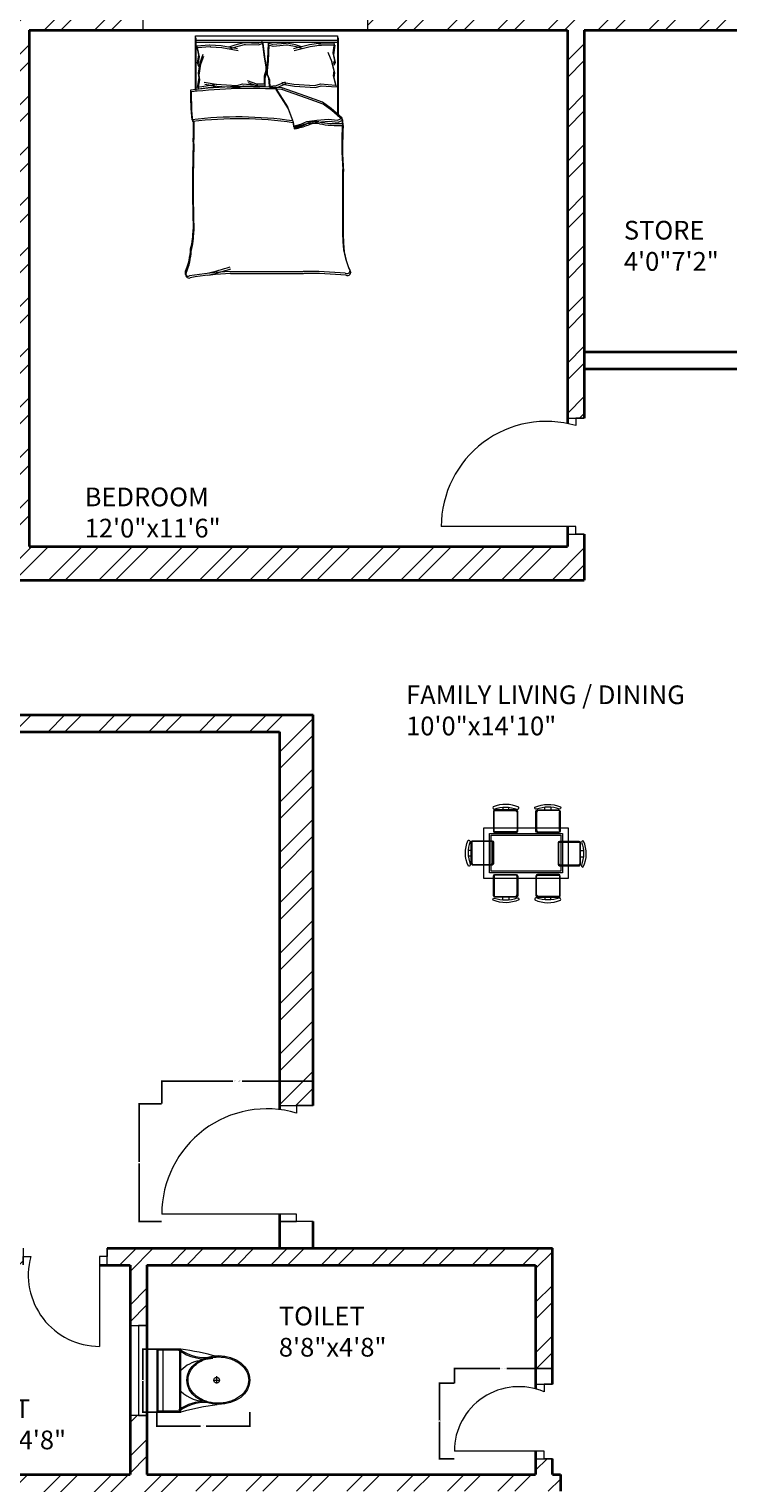
# Model space of a CAD drawing. Units: inches. Extents: x 1152 to 2588, y 1459 to 2618.
# Tile 5 of 17: x 1378 to 1565, y 1843 to 2231. Entities that reach past the tile are written whole.
import ezdxf

# ---------------------------------------------------------------- set-up
doc = ezdxf.new("R2010")
doc.units = ezdxf.units.IN
for name, color, linetype, lineweight in [('A-ANNO-DIMS', 2, 'Continuous', 18), ('A-AREA-IDEN', 7, 'Continuous', 18), ('A-DOOR', 4, 'Continuous', 18), ('A-FLOR-FIXT', 9, 'Continuous', 18), ('A-FURN', 8, 'Continuous', 13), ('A-GLAZ', 4, 'Continuous', 18), ('A-WALL', 7, 'Continuous', 35), ('A-WALL-PATT', 8, 'Continuous', 13)]:
    doc.layers.add(name, color=color, linetype=linetype, lineweight=lineweight)
doc.styles.get("Standard").update_dxf_attribs({"font": 'arial.ttf'})
doc.dimstyles.get("Standard").update_dxf_attribs({"dimtxt": 0.18, "dimasz": 0.18, "dimexe": 0.18, "dimexo": 0.0625, "dimgap": 0.09, "dimtad": 0, "dimtih": 1, "dimtoh": 1, "dimdec": 4, "dimzin": 0, "dimdsep": 46, "dimtxsty": 'Standard', "dimcen": 0.09, "dimadec": 0, "dimazin": 0, "dimtfac": 1, "dimtdec": 4, "dimtofl": 0, "dimtmove": 0, "dimatfit": 3, "dimfxl": 1, "dimtolj": 1, "dimtzin": 0, "dimarcsym": 0})

# ---------------------------------------------------------------- blocks, each defined once
blk = doc.blocks.new('A$C31115884')
for p, q in [((283, 498), (223, 498)), ((258, 466), (258, 523)), ((0, 200), (0, 0)), ((520, 200), (0, 200)), ((10, 190), (10, 10)), ((510, 190), (10, 190)), ((510, 10), (510, 190)), ((520, 0), (520, 200)), ((510, 54), (0, 54)), ((10, 10), (510, 10)), ((0, 0), (520, 0))]:
    blk.add_line(p, q)
blk.add_circle((256, 496), 23.6)
for centre, radius, start, end in [((2778, -205), 2807, 165.4549, 171.7133), ((3237, 905), 2807, 188.2867, 194.5451), ((-295, 403), 365, 324.2091, 9.3499), ((-295, 403), 375, 324.2091, 9.3499), ((139, 406), 293, 315.8436, 2.6563), ((806, 403), 375, 179.2036, 215.7909), ((806, 403), 365, 170.6501, 215.7909), ((384, 406), 293, 190.2774, 224.1564)]:
    blk.add_arc(centre, radius, start, end)
blk.add_ellipse((256, 510), major_axis=(0, -261), ratio=0.772727)
blk.add_open_spline([(256, 259), (263, 259), (270, 260), (288, 262), (299, 265), (320, 273), (330, 278), (350, 291), (360, 299), (378, 316), (386, 326), (402, 347), (409, 358), (421, 383), (427, 395), (436, 422), (440, 436), (445, 465), (447, 480), (448, 509), (448, 524), (445, 553), (443, 568), (436, 596), (432, 610), (422, 636), (416, 649), (402, 672), (395, 683), (379, 703), (370, 712), (351, 728), (341, 735), (321, 746), (310, 751), (289, 757), (278, 759), (256, 761), (245, 761), (223, 757), (212, 754), (191, 746), (181, 741), (161, 728), (151, 720), (133, 703), (125, 693), (110, 672), (103, 660), (90, 636), (85, 623), (76, 596), (72, 582), (67, 553), (66, 538), (64, 509), (65, 494), (68, 465), (70, 450), (77, 422), (81, 408), (91, 382), (97, 370), (111, 346), (118, 335), (135, 316), (144, 307), (162, 291), (172, 284), (193, 273), (203, 269), (225, 262), (236, 260), (250, 259), (253, 259), (256, 259)], degree=3, knots=[0, 0, 0, 0, 0.110105, 0.110105, 0.285049, 0.285049, 0.459994, 0.459994, 0.634938, 0.634938, 0.809882, 0.809882, 0.984827, 0.984827, 1.159771, 1.159771, 1.334715, 1.334715, 1.50966, 1.50966, 1.684604, 1.684604, 1.859549, 1.859549, 2.034493, 2.034493, 2.209437, 2.209437, 2.384382, 2.384382, 2.559326, 2.559326, 2.73427, 2.73427, 2.909215, 2.909215, 3.084159, 3.084159, 3.259103, 3.259103, 3.434048, 3.434048, 3.608992, 3.608992, 3.783936, 3.783936, 3.958881, 3.958881, 4.133825, 4.133825, 4.30877, 4.30877, 4.483714, 4.483714, 4.658658, 4.658658, 4.833603, 4.833603, 5.008547, 5.008547, 5.183491, 5.183491, 5.358436, 5.358436, 5.53338, 5.53338, 5.708324, 5.708324, 5.883269, 5.883269, 6.058213, 6.058213, 6.233158, 6.233158, 6.283185, 6.283185, 6.283185, 6.283185])
blk = doc.blocks.new('BED-PLAN')
for p, q in [((49.83, 41.36), (64.23, 41.36)), ((49.83, 41.36), (64.23, 41.36)), ((50.34, 41.54), (64.74, 41.54)), ((50.34, 41.54), (64.74, 41.54)), ((51.02, 36.75), (50.45, 40.8)), ((50.45, 40.8), (52.97, 40.34)), ((51.02, 36.75), (50.45, 40.8)), ((50.45, 40.8), (52.97, 40.34)), ((51.53, 36.93), (50.95, 40.98)), ((50.95, 40.98), (53.48, 40.52)), ((51.53, 36.93), (50.95, 40.98)), ((50.95, 40.98), (53.48, 40.52)), ((51.81, 39.05), (51.28, 35.85)), ((51.81, 39.05), (51.28, 35.85)), ((52.32, 39.23), (51.79, 36.03)), ((52.32, 39.23), (51.79, 36.03)), ((52.97, 40.34), (54.24, 40.57)), ((52.97, 40.34), (54.24, 40.57)), ((53.48, 40.52), (54.75, 40.75)), ((53.48, 40.52), (54.75, 40.75)), ((54.24, 40.57), (57.11, 40.11)), ((54.24, 40.57), (57.11, 40.11)), ((54.75, 40.75), (57.62, 40.29)), ((54.75, 40.75), (57.62, 40.29)), ((57, 40.91), (56.19, 40.45)), ((57, 40.91), (56.19, 40.45)), ((57.51, 41.09), (56.7, 40.64)), ((57.51, 41.09), (56.7, 40.64)), ((59.07, 40.57), (57, 40.91)), ((59.07, 40.57), (57, 40.91)), ((57.11, 40.11), (59.3, 39.3)), ((57.11, 40.11), (59.3, 39.3)), ((59.57, 40.75), (57.51, 41.09)), ((59.57, 40.75), (57.51, 41.09)), ((57.62, 40.29), (59.8, 39.49)), ((57.62, 40.29), (59.8, 39.49)), ((61.59, 41.03), (59.07, 40.57)), ((61.59, 41.03), (59.07, 40.57)), ((62.1, 41.21), (59.57, 40.75)), ((62.1, 41.21), (59.57, 40.75)), ((61.58, 41.03), (61.84, 37.62)), ((61.58, 41.02), (61.84, 37.62)), ((62.08, 41.21), (62.35, 37.8)), ((62.08, 41.21), (62.35, 37.8)), ((63.01, 41.36), (63.01, 3.37)), ((63.01, 41.36), (63.01, 3.37)), ((63.52, 41.54), (63.52, 3.56)), ((63.52, 41.54), (63.52, 3.56)), ((64.74, 41.54), (64.74, 3.56)), ((51.28, 35.85), (50.93, 30.27)), ((51.28, 35.85), (50.93, 30.27)), ((51.28, 35.85), (51.02, 36.75)), ((51.28, 35.85), (51.02, 36.75)), ((51.79, 36.03), (51.44, 30.46)), ((51.79, 36.03), (51.44, 30.46)), ((51.79, 36.03), (51.53, 36.93)), ((51.79, 36.03), (51.53, 36.93)), ((61.82, 37.54), (61.59, 34.5)), ((61.82, 37.54), (61.59, 34.5)), ((61.84, 37.62), (61.82, 37.54)), ((61.84, 37.62), (61.82, 37.54)), ((62.33, 37.72), (62.1, 34.68)), ((62.33, 37.72), (62.1, 34.68)), ((62.35, 37.8), (62.33, 37.72)), ((62.35, 37.8), (62.33, 37.72)), ((1.24, 32.15), (1.24, 12.59)), ((1.24, 32.15), (1.24, 12.59)), ((1.75, 32.33), (1.75, 12.77)), ((1.75, 32.33), (1.75, 12.77)), ((61.59, 34.5), (60.79, 30.13)), ((61.59, 34.5), (60.79, 30.13)), ((61.25, 32.32), (61.82, 30.71)), ((61.25, 32.32), (61.82, 30.71)), ((62.1, 34.68), (61.3, 30.31)), ((62.1, 34.68), (61.3, 30.31)), ((61.76, 32.5), (62.33, 30.89)), ((61.76, 32.5), (62.33, 30.89)), ((50.93, 30.27), (51.38, 28.72)), ((50.93, 30.27), (51.38, 28.72)), ((51.38, 28.72), (51.06, 24.64)), ((51.38, 28.72), (51.06, 24.64)), ((51.3, 24.96), (52.17, 27.46)), ((51.3, 24.96), (52.17, 27.46)), ((51.44, 30.46), (51.89, 28.9)), ((51.44, 30.46), (51.89, 28.9)), ((51.89, 28.9), (51.56, 24.82)), ((51.89, 28.9), (51.56, 24.82)), ((51.81, 25.15), (52.68, 27.65)), ((51.81, 25.15), (52.68, 27.65)), ((61.82, 30.71), (62.4, 28.41)), ((61.82, 30.71), (62.4, 28.41)), ((62.4, 28.15), (62.28, 24.62)), ((62.4, 28.15), (62.28, 24.62)), ((62.33, 30.89), (62.91, 28.59)), ((62.33, 30.89), (62.91, 28.59)), ((62.4, 28.41), (62.4, 28.15)), ((62.4, 28.41), (62.4, 28.15)), ((62.91, 28.34), (62.79, 24.8)), ((62.91, 28.34), (62.79, 24.8)), ((62.91, 28.59), (62.91, 28.34)), ((62.91, 28.59), (62.91, 28.34)), ((51.3, 23.01), (51.3, 24.96)), ((51.3, 23.01), (51.3, 24.96)), ((51.81, 23.19), (51.81, 25.15)), ((51.81, 23.19), (51.81, 25.15)), ((62.74, 23.47), (58.49, 23.01)), ((62.74, 23.47), (58.49, 23.01)), ((63.25, 23.65), (59, 23.19)), ((63.25, 23.65), (59, 23.19)), ((62.28, 24.62), (62.74, 23.47)), ((62.28, 24.62), (62.74, 23.47)), ((62.79, 24.8), (63.25, 23.65)), ((62.79, 24.8), (63.25, 23.65)), ((50.41, 20.07), (45.25, 16.74)), ((50.41, 20.07), (45.25, 16.74)), ((50.92, 20.25), (45.76, 16.92)), ((50.92, 20.25), (45.76, 16.92)), ((52.93, 21.76), (50.8, 21.63)), ((52.93, 21.76), (50.8, 21.63)), ((50.8, 21.63), (50.92, 19.68)), ((50.8, 21.63), (50.92, 19.68)), ((50.92, 19.68), (51.95, 17.24)), ((50.92, 19.68), (51.95, 17.24)), ((53.43, 23.01), (51.3, 23.01)), ((53.43, 23.01), (51.3, 23.01)), ((53.44, 21.95), (51.31, 21.81)), ((53.44, 21.94), (51.31, 21.81)), ((51.31, 21.81), (51.43, 19.86)), ((51.31, 21.81), (51.43, 19.86)), ((51.43, 19.86), (52.45, 17.42)), ((51.43, 19.86), (52.45, 17.42)), ((53.94, 23.19), (51.81, 23.19)), ((53.94, 23.19), (51.81, 23.19)), ((54.39, 22.32), (52.93, 21.76)), ((54.39, 22.32), (52.93, 21.76)), ((54.93, 22.55), (53.43, 23.01)), ((54.93, 22.55), (53.43, 23.01)), ((54.9, 22.5), (53.44, 21.94)), ((54.9, 22.5), (53.44, 21.95)), ((55.44, 22.73), (53.94, 23.19)), ((55.44, 22.73), (53.94, 23.19)), ((55.42, 22.38), (54.39, 22.32)), ((55.42, 22.38), (54.39, 22.32)), ((55.93, 22.56), (54.9, 22.5)), ((55.93, 22.56), (54.9, 22.5)), ((55.96, 22.55), (54.93, 22.55)), ((55.96, 22.55), (54.93, 22.55)), ((57.98, 22.08), (55.42, 22.38)), ((57.98, 22.08), (55.42, 22.38)), ((56.47, 22.73), (55.44, 22.73)), ((56.47, 22.73), (55.44, 22.73)), ((58.48, 22.26), (55.93, 22.56)), ((58.48, 22.26), (55.93, 22.56)), ((58.49, 23.01), (55.96, 22.55)), ((58.49, 23.01), (55.96, 22.55)), ((59, 23.19), (56.47, 22.73)), ((59, 23.19), (56.47, 22.73)), ((62.25, 21.89), (57.98, 22.08)), ((62.25, 21.89), (57.98, 22.08)), ((62.76, 22.07), (58.48, 22.26)), ((62.76, 22.07), (58.48, 22.26)), ((61.86, 20.71), (62.25, 21.89)), ((61.86, 20.71), (62.25, 21.89)), ((62.2, 17.19), (61.86, 20.71)), ((62.2, 17.19), (61.86, 20.71)), ((62.37, 20.89), (62.76, 22.07)), ((62.37, 20.89), (62.76, 22.07)), ((62.71, 17.37), (62.37, 20.89)), ((62.71, 17.37), (62.37, 20.89)), ((42.19, 15.57), (40.59, 15.32)), ((42.19, 15.57), (40.59, 15.32)), ((45.25, 16.74), (41.68, 15.39)), ((45.25, 16.74), (41.68, 15.39)), ((45.76, 16.92), (42.19, 15.57)), ((45.76, 16.92), (42.19, 15.57)), ((48.08, 11.82), (50.41, 18.44)), ((48.08, 11.82), (50.41, 18.44)), ((48.59, 12), (50.92, 18.63)), ((48.59, 12), (50.92, 18.63)), ((51.81, 18.24), (51.28, 15.03)), ((51.81, 18.24), (51.28, 15.03)), ((52.32, 18.42), (51.79, 15.22)), ((52.32, 18.42), (51.79, 15.22)), ((61.78, 14.61), (62.21, 16.94)), ((61.78, 14.61), (62.21, 16.94)), ((62.21, 16.94), (62.2, 17.19)), ((62.21, 16.94), (62.2, 17.19)), ((62.29, 14.79), (62.72, 17.12)), ((62.29, 14.79), (62.72, 17.12)), ((62.72, 17.12), (62.71, 17.37)), ((62.72, 17.12), (62.71, 17.37)), ((41.68, 15.39), (40.08, 15.14)), ((41.68, 15.39), (40.08, 15.14)), ((40.08, 15.14), (40.58, 13.17)), ((40.08, 15.14), (40.58, 13.17)), ((40.58, 13.17), (41.31, 11.57)), ((40.58, 13.17), (41.31, 11.57)), ((40.59, 15.32), (41.08, 13.35)), ((40.59, 15.32), (41.08, 13.35)), ((41.08, 13.35), (41.82, 11.75)), ((41.08, 13.35), (41.82, 11.75)), ((41.82, 11.75), (42.19, 9.04)), ((41.82, 11.75), (42.19, 9.04)), ((46.48, 7.38), (48.08, 11.82)), ((46.48, 7.38), (48.08, 11.82)), ((46.99, 7.57), (48.59, 12)), ((46.99, 7.57), (48.59, 12)), ((51.28, 15.03), (50.93, 9.46)), ((51.28, 15.03), (50.93, 9.46)), ((51.79, 15.22), (51.44, 9.64)), ((51.79, 15.22), (51.44, 9.64)), ((61.79, 10.81), (60.71, 15.11)), ((61.79, 10.81), (60.71, 15.11)), ((62.3, 10.99), (61.22, 15.3)), ((62.3, 10.99), (61.22, 15.3)), ((61.31, 12.96), (61.78, 14.61)), ((61.31, 12.96), (61.78, 14.61)), ((61.82, 13.15), (62.29, 14.79)), ((61.82, 13.15), (62.29, 14.79)), ((41.31, 11.57), (41.68, 8.86)), ((41.31, 11.57), (41.68, 8.86)), ((41.68, 8.86), (41.93, 5.78)), ((41.68, 8.86), (41.93, 5.78)), ((42.19, 9.04), (42.44, 5.97)), ((42.19, 9.04), (42.44, 5.97)), ((50.93, 9.46), (51.38, 7.9)), ((50.93, 9.46), (51.38, 7.9)), ((51.38, 7.9), (51.06, 3.82)), ((51.38, 7.9), (51.06, 3.82)), ((51.44, 9.64), (51.89, 8.09)), ((51.44, 9.64), (51.89, 8.09)), ((51.89, 8.09), (51.56, 4.01)), ((51.89, 8.09), (51.56, 4.01)), ((62.21, 7.79), (61.79, 10.81)), ((62.21, 7.79), (61.79, 10.81)), ((62.2, 4.29), (62.27, 8.59)), ((62.2, 4.29), (62.27, 8.58)), ((62.27, 8.59), (62.21, 7.79)), ((62.27, 8.58), (62.21, 7.79)), ((62.72, 7.97), (62.3, 10.99)), ((62.72, 7.97), (62.3, 10.99)), ((62.71, 4.47), (62.78, 8.77)), ((62.71, 4.47), (62.78, 8.77)), ((62.78, 8.77), (62.72, 7.97)), ((62.78, 8.77), (62.72, 7.97)), ((41.93, 5.78), (41.68, 3.32)), ((41.93, 5.78), (41.68, 3.32)), ((42.18, 2.1), (44.76, 5.05)), ((42.18, 2.1), (44.76, 5.05)), ((42.44, 5.97), (42.19, 3.5)), ((42.44, 5.97), (42.19, 3.5)), ((42.68, 2.28), (45.27, 5.23)), ((42.68, 2.28), (45.27, 5.23)), ((44.76, 5.05), (46.48, 7.38)), ((44.76, 5.05), (46.48, 7.38)), ((45.27, 5.23), (46.99, 7.57)), ((45.27, 5.23), (46.99, 7.57)), ((51.06, 3.82), (53.55, 4.44)), ((51.06, 3.82), (53.55, 4.44)), ((51.56, 4.01), (54.06, 4.62)), ((51.56, 4.01), (54.06, 4.62)), ((53.55, 4.44), (54.83, 4.29)), ((53.55, 4.44), (54.83, 4.29)), ((54.06, 4.62), (55.34, 4.47)), ((54.06, 4.62), (55.34, 4.47)), ((54.83, 4.29), (57.67, 4.93)), ((54.83, 4.29), (57.67, 4.93)), ((55.34, 4.47), (58.17, 5.11)), ((55.34, 4.47), (58.17, 5.11)), ((57.6, 4.12), (56.77, 4.53)), ((57.6, 4.12), (56.77, 4.53)), ((58.11, 4.3), (57.28, 4.71)), ((58.11, 4.3), (57.28, 4.71)), ((59.65, 4.59), (57.6, 4.12)), ((59.65, 4.59), (57.6, 4.12)), ((57.67, 4.93), (59.8, 5.87)), ((57.67, 4.93), (59.8, 5.87)), ((60.15, 4.77), (58.11, 4.3)), ((60.15, 4.77), (58.11, 4.3)), ((58.17, 5.11), (60.3, 6.05)), ((58.17, 5.11), (60.3, 6.05)), ((62.2, 4.29), (59.65, 4.59)), ((62.2, 4.29), (59.65, 4.59)), ((62.71, 4.47), (60.15, 4.77)), ((62.71, 4.47), (60.15, 4.77)), ((40.79, 2.04), (42.18, 2.1, 3.08)), ((40.79, 2.04), (42.18, 2.1, 3.08)), ((41.3, 2.22), (42.68, 2.28, 3.08)), ((41.3, 2.22), (42.68, 2.28, 3.08)), ((41.68, 3.32), (42.18, 2.1)), ((41.68, 3.32), (42.18, 2.1)), ((42.19, 3.5), (42.68, 2.28)), ((42.19, 3.5), (42.68, 2.28)), ((64.23, 3.37), (43.08, 3.37)), ((64.23, 3.37), (43.08, 3.37)), ((64.74, 3.56), (43.59, 3.56)), ((64.74, 3.56), (43.59, 3.56))]:
    blk.add_line(p, q)
for centre, radius, start, end in [((0.86, 43.26), 0.866, 56.1736, 203.4781), ((0.86, 43.26), 0.866, 56.1736, 203.4781), ((-95.41, 27.09), 96.78, 2.9958, 9.4091), ((-95.41, 27.09), 96.78, 2.9958, 9.4091), ((1.37, 43.44), 0.866, 56.1736, 203.4781), ((1.37, 43.44), 0.866, 56.1736, 203.4781), ((-94.9, 27.27), 96.78, 2.9958, 9.4091), ((-94.9, 27.27), 96.78, 2.9958, 9.4091), ((8.37, 61.34), 18.73, 247.9751, 266.652), ((8.37, 61.34), 18.73, 247.9751, 266.652), ((8.88, 61.52), 18.73, 247.9751, 266.652), ((8.88, 61.52), 18.73, 247.9751, 266.652), ((13.46, 65.69), 23.56, 256.0648, 268.9113), ((13.46, 65.69), 23.56, 256.0648, 268.9113), ((48.76, -23.39), 66.22, 88.7218, 95.604), ((48.76, -23.39), 66.22, 88.7218, 95.604), ((-79.97, 27.33), 131.13, 356.0865, 6.7821), ((-79.97, 27.33), 131.13, 356.0865, 6.7821), ((12.95, 65.51), 23.56, 256.0648, 268.9113), ((12.95, 65.51), 23.56, 256.0648, 268.9113), ((24, -341.25), 383.38, 88.2277, 91.7185), ((24, -341.25), 383.38, 88.2277, 91.7185), ((24.51, -341.07), 383.38, 88.2277, 91.7185), ((24.51, -341.07), 383.38, 88.2277, 91.7185), ((39.45, 177.11), 135.22, 268.4762, 271.0082), ((39.45, 177.11), 135.22, 268.4762, 271.0082), ((39.96, 177.3), 135.22, 268.4762, 271.0082), ((39.96, 177.3), 135.22, 268.4762, 271.0082), ((-60.02, 30.01), 102.56, 351.7845, 6.9006), ((-60.02, 30.01), 102.56, 351.7845, 6.9006), ((48.26, -23.57), 66.22, 88.7218, 95.604), ((48.26, -23.57), 66.22, 88.7218, 95.604), ((-59.52, 30.19), 102.56, 351.7845, 6.9006), ((-59.52, 30.19), 102.56, 351.7845, 6.9006), ((-80.48, 27.15), 131.13, 356.0865, 6.7821), ((-80.48, 27.15), 131.13, 356.0865, 6.7821), ((83.08, 57.81), 84.62, 193.3832, 197.7053), ((83.08, 57.81), 84.62, 193.3832, 197.7053), ((83.59, 57.99), 84.62, 193.3832, 197.7053), ((83.59, 57.99), 84.62, 193.3832, 197.7053), ((-104.51, 11.41), 105.75, 354.4998, 0.6351), ((-104.51, 11.41), 105.75, 354.4998, 0.6351), ((-104, 11.59), 105.75, 354.4998, 0.6351), ((-104, 11.59), 105.75, 354.4998, 0.6351), ((40.03, 15), 0.147, 70.2464, 181.1377), ((40.03, 15), 0.147, 70.2464, 181.1377), ((63.05, 19.36), 23.57, 190.6617, 199.8806), ((63.05, 19.36), 23.57, 190.6617, 199.8806), ((40.54, 15.18), 0.147, 70.2464, 181.1377), ((40.54, 15.18), 0.147, 70.2464, 181.1377), ((63.56, 19.54), 23.57, 190.6617, 199.8806), ((63.56, 19.54), 23.57, 190.6617, 199.8806), ((69.52, 3.32), 28.76, 169.8763, 182.5657), ((69.52, 3.32), 28.76, 169.8763, 182.5657), ((36.36, 9.35), 4.95, 348.6608, 23.7384), ((36.36, 9.35), 4.95, 348.6608, 23.7384), ((70.03, 3.51), 28.76, 169.8763, 182.5657), ((70.03, 3.51), 28.76, 169.8763, 182.5657), ((36.86, 9.53), 4.95, 348.6608, 23.7384), ((36.86, 9.53), 4.95, 348.6608, 23.7384), ((1.54, 0.87), 0.876, 152.6588, 266.02), ((1.54, 0.87), 0.876, 152.6588, 266.02), ((2.05, 1.06), 0.876, 152.6588, 266.02), ((2.05, 1.06), 0.876, 152.6588, 266.02), ((9.65, -16.41), 18.33, 87.4714, 116.4681), ((9.65, -16.41), 18.33, 87.4714, 116.4681), ((10.16, -16.23), 18.33, 87.4714, 116.4681), ((10.16, -16.23), 18.33, 87.4714, 116.4681), ((10.32, 3628.06), 3626.16, 270.00217, 270.28689), ((10.32, 3628.06), 3626.16, 270.00217, 270.28689), ((10.83, 3628.24), 3626.16, 270.00217, 270.28689), ((10.83, 3628.24), 3626.16, 270.00217, 270.28689), ((35.36, -100.76), 102.94, 86.9791, 93.8365), ((35.36, -100.76), 102.94, 86.9791, 93.8365), ((35.87, -100.58), 102.94, 86.9791, 93.8365), ((35.87, -100.57), 102.94, 86.9791, 93.8365)]:
    blk.add_arc(centre, radius, start, end)
blk = doc.blocks.new('DOOR-36-BED-NORTH')
for p, q in [((33.75, 30.96), (38.25, 30.96)), ((38.25, 30.96), (36, 30.96)), ((36, 30.96), (36, 28.96)), ((36, 2), (0, 2)), ((36, 0), (36, 2)), ((33.75, 0), (38.25, 0)), ((38.25, 0), (36, 0))]:
    blk.add_line(p, q)
blk.add_arc((28.09, 2), 28.09, 73.6552, 180)
blk = doc.blocks.new('DOOR-36-BED-WEST')
for p, q in [((31.5, 31), (40.5, 31)), ((40.5, 31), (36, 31)), ((36, 31), (36, 29)), ((36, 2), (0, 2)), ((36, 0), (36, 2)), ((40.5, 0), (31.5, 0)), ((31.5, 0), (36, 0))]:
    blk.add_line(p, q)
blk.add_arc((28.13, 2), 28.13, 73.7471, 180)
blk = doc.blocks.new('DOOR-24-BATH-WEST')
for p, q in [((0, 26.25), (0, 21.75)), ((0, 21.75), (0, 24)), ((0, 24), (2, 24)), ((22.43, 24), (20.43, 24)), ((20.43, 24), (20.43, 0)), ((22.43, 21.75), (22.43, 26.25)), ((22.43, 26.25), (22.43, 24))]:
    blk.add_line(p, q)
blk.add_arc((20.43, 19.08), 19.08, 165.0504, 270)
blk = doc.blocks.new('DOOR-24-BATH-CENTRE')
for p, q in [((21.75, 19.88), (26.25, 19.88)), ((26.25, 19.88), (24, 19.88)), ((24, 19.88), (24, 17.88)), ((24, 2), (0, 2)), ((24, 0), (24, 2)), ((21.75, 0), (26.25, 0)), ((26.25, 0), (24, 0))]:
    blk.add_line(p, q)
blk.add_arc((17.25, 2), 17.25, 66.9754, 180)
blk = doc.blocks.new('WIN-24-INTERIOR')
for p, q in [((0, 24), (4.5, 24)), ((4.5, 24), (2.25, 24)), ((2.25, 24), (2.25, 0)), ((4.5, 0), (0, 0)), ((2.25, 0), (4.5, 0))]:
    blk.add_line(p, q)
blk = doc.blocks.new('WIN-60-BED-NORTH')
for p, q in [((0, 0), (0, 9)), ((0, 9), (0, 4.5)), ((60, 4.5), (60, 9)), ((60, 9), (60, 0)), ((0, 4.5), (60, 4.5))]:
    blk.add_line(p, q)
blk = doc.blocks.new('*D24')
at = {"layer": 'A-ANNO-DIMS', "color": 0, "lineweight": -2, "transparency": 16777216}
for p, q in [((1492.17, 1869.5), (1492.17, 1873.55)), ((1492.35, 1873.37), (1504.36, 1873.37)), ((1518.24, 1873.37), (1506.23, 1873.37)), ((1518.42, 1869.5), (1518.42, 1873.55))]:
    blk.add_line(p, q, dxfattribs=at)
at = {"layer": 'A-ANNO-DIMS', "color": 0, "transparency": 16777216}
for points in [[(1492.35, 1873.4), (1492.35, 1873.34), (1492.17, 1873.37)], [(1518.24, 1873.4), (1518.24, 1873.34), (1518.42, 1873.37)]]:
    blk.add_solid(points, dxfattribs=at)
at = {"layer": 'Defpoints', "color": 0, "transparency": 16777216}
for p in [(1518.42, 1873.37), (1492.17, 1869.44), (1518.42, 1869.44)]:
    blk.add_point(p, dxfattribs=at)
at = {"layer": 'A-ANNO-DIMS', "color": 0, "transparency": 16777216, "insert": (1505.29, 1873.37), "char_height": 0.18, "attachment_point": 5}
blk.add_mtext('\\A1;DOOR 26 TYP.', dxfattribs=at)
blk = doc.blocks.new('*D25')
at = {"layer": 'A-ANNO-DIMS', "color": 0, "lineweight": -2, "transparency": 16777216}
for p, q in [((1492.1, 1869.44), (1488.05, 1869.44)), ((1488.23, 1869.26), (1488.23, 1859.55)), ((1488.23, 1849.47), (1488.23, 1859.18)), ((1492.1, 1849.29), (1488.05, 1849.29))]:
    blk.add_line(p, q, dxfattribs=at)
at = {"layer": 'A-ANNO-DIMS', "color": 0, "transparency": 16777216}
for points in [[(1488.2, 1869.26), (1488.26, 1869.26), (1488.23, 1869.44)], [(1488.2, 1849.47), (1488.26, 1849.47), (1488.23, 1849.29)]]:
    blk.add_solid(points, dxfattribs=at)
at = {"layer": 'Defpoints', "color": 0, "transparency": 16777216}
for p in [(1488.23, 1869.44), (1492.17, 1869.44), (1492.17, 1849.29)]:
    blk.add_point(p, dxfattribs=at)
at = {"layer": 'A-ANNO-DIMS', "color": 0, "transparency": 16777216, "insert": (1488.23, 1859.36), "char_height": 0.18, "attachment_point": 5}
blk.add_mtext('\\A1;20 TYP.', dxfattribs=at)
blk = doc.blocks.new('*D30')
at = {"layer": 'A-ANNO-DIMS', "color": 0, "lineweight": -2, "transparency": 16777216}
for p, q in [((1412.55, 1861.69), (1412.55, 1857.84)), ((1437.48, 1861.69), (1437.48, 1857.84)), ((1412.73, 1858.02), (1424.24, 1858.02)), ((1437.3, 1858.02), (1425.79, 1858.02))]:
    blk.add_line(p, q, dxfattribs=at)
at = {"layer": 'A-ANNO-DIMS', "color": 0, "transparency": 16777216}
for points in [[(1412.73, 1858.05), (1412.73, 1857.99), (1412.55, 1858.02)], [(1437.3, 1858.05), (1437.3, 1857.99), (1437.48, 1858.02)]]:
    blk.add_solid(points, dxfattribs=at)
at = {"layer": 'Defpoints', "color": 0, "transparency": 16777216}
for p in [(1412.55, 1861.76), (1437.48, 1861.76), (1437.48, 1858.02)]:
    blk.add_point(p, dxfattribs=at)
at = {"layer": 'A-ANNO-DIMS', "color": 0, "transparency": 16777216, "insert": (1425.01, 1858.02), "char_height": 0.18, "attachment_point": 5}
blk.add_mtext('\\A1;WC 25 TYP.', dxfattribs=at)
blk = doc.blocks.new('*D31')
at = {"layer": 'A-ANNO-DIMS', "color": 0, "lineweight": -2, "transparency": 16777216}
for p, q in [((1412.49, 1878.58), (1408.63, 1878.58)), ((1408.81, 1878.4), (1408.81, 1870.35)), ((1408.81, 1861.94), (1408.81, 1869.99)), ((1412.49, 1861.76), (1408.63, 1861.76))]:
    blk.add_line(p, q, dxfattribs=at)
at = {"layer": 'A-ANNO-DIMS', "color": 0, "transparency": 16777216}
for points in [[(1408.78, 1878.4), (1408.84, 1878.4), (1408.81, 1878.58)], [(1408.78, 1861.94), (1408.84, 1861.94), (1408.81, 1861.76)]]:
    blk.add_solid(points, dxfattribs=at)
at = {"layer": 'Defpoints', "color": 0, "transparency": 16777216}
for p in [(1412.55, 1878.58), (1408.81, 1861.76), (1412.55, 1861.76)]:
    blk.add_point(p, dxfattribs=at)
at = {"layer": 'A-ANNO-DIMS', "color": 0, "transparency": 16777216, "insert": (1408.81, 1870.17), "char_height": 0.18, "attachment_point": 5}
blk.add_mtext('\\A1;17 TYP.', dxfattribs=at)
blk = doc.blocks.new('*D42')
at = {"layer": 'A-ANNO-DIMS', "color": 0, "lineweight": -2, "transparency": 16777216}
for p, q in [((1413.92, 1944.19), (1413.92, 1950.38)), ((1414.1, 1950.2), (1432.94, 1950.2)), ((1454.24, 1950.2), (1435.4, 1950.2)), ((1454.42, 1944.19), (1454.42, 1950.38))]:
    blk.add_line(p, q, dxfattribs=at)
at = {"layer": 'A-ANNO-DIMS', "color": 0, "transparency": 16777216}
for points in [[(1414.1, 1950.23), (1414.1, 1950.17), (1413.92, 1950.2)], [(1454.24, 1950.23), (1454.24, 1950.17), (1454.42, 1950.2)]]:
    blk.add_solid(points, dxfattribs=at)
at = {"layer": 'Defpoints', "color": 0, "transparency": 16777216}
for p in [(1454.42, 1950.2), (1413.92, 1944.13), (1454.42, 1944.13)]:
    blk.add_point(p, dxfattribs=at)
at = {"layer": 'A-ANNO-DIMS', "color": 0, "transparency": 16777216, "insert": (1434.17, 1950.2), "char_height": 0.18, "attachment_point": 5}
blk.add_mtext('\\A1;BED DOOR 41 TYP.', dxfattribs=at)
blk = doc.blocks.new('*D43')
at = {"layer": 'A-ANNO-DIMS', "color": 0, "lineweight": -2, "transparency": 16777216}
for p, q in [((1413.85, 1944.13), (1407.66, 1944.13)), ((1407.84, 1943.95), (1407.84, 1928.57)), ((1407.84, 1912.83), (1407.84, 1928.21)), ((1413.85, 1912.65), (1407.66, 1912.65))]:
    blk.add_line(p, q, dxfattribs=at)
at = {"layer": 'A-ANNO-DIMS', "color": 0, "transparency": 16777216}
for points in [[(1407.81, 1943.95), (1407.87, 1943.95), (1407.84, 1944.13)], [(1407.81, 1912.83), (1407.87, 1912.83), (1407.84, 1912.65)]]:
    blk.add_solid(points, dxfattribs=at)
at = {"layer": 'Defpoints', "color": 0, "transparency": 16777216}
for p in [(1407.84, 1944.13), (1413.92, 1944.13), (1413.92, 1912.65)]:
    blk.add_point(p, dxfattribs=at)
at = {"layer": 'A-ANNO-DIMS', "color": 0, "transparency": 16777216, "insert": (1407.84, 1928.39), "char_height": 0.18, "attachment_point": 5}
blk.add_mtext('\\A1;31 TYP.', dxfattribs=at)

msp = doc.modelspace()

# ---------------------------------------------------------------- hatches: boundary and pattern name
at = {"layer": 'A-WALL-PATT'}
h = msp.add_hatch(dxfattribs=at)
h.set_pattern_fill('ANSI32', color=256)
h.paths.add_polyline_path([(1408.9272, 2240.0458), (1276.4165, 2240.0458), (1276.4165, 2192.7491), (1285.4165, 2192.7491), (1285.4165, 2231.0458), (1369.4165, 2231.0458), (1369.4165, 2084.0458), (1526.9165, 2084.0458), (1526.9165, 2096.3728), (1524.6665, 2096.3728), (1522.4165, 2096.3728), (1522.4165, 2093.0458), (1378.4165, 2093.0458), (1378.4165, 2231.0458), (1408.9272, 2231.0458)])
h.paths.add_polyline_path([(1736.4165, 2240.0458), (1468.9272, 2240.0458), (1468.9272, 2231.0458), (1522.4165, 2231.0458), (1522.4165, 2127.3313), (1526.9165, 2127.3313), (1526.9165, 2231.0458), (1574.9165, 2231.0458), (1574.9165, 2188.0458), (1579.4165, 2188.0458), (1579.4165, 2231.0458), (1727.4165, 2231.0458), (1727.4165, 2183.9728), (1736.4165, 2183.9728)])
h.paths.add_polyline_path([(1285.4165, 2156.7491), (1276.4165, 2156.7491), (1276.4165, 2084.0458), (1285.4165, 2084.0458)], flags=17)
h.paths.add_polyline_path([(1285.4165, 2043.5458), (1445.4165, 2043.5458), (1445.4165, 1943.6503), (1454.4165, 1943.6503), (1454.4165, 2048.0458), (1276.4165, 2048.0458), (1276.4165, 2019.2077), (1280.9165, 2019.2077), (1285.4165, 2019.2077)])
h.paths.add_polyline_path([(1285.4165, 1959.2077), (1276.4165, 1959.2077), (1276.4165, 1891.1319), (1280.9165, 1891.1319), (1285.4165, 1891.1319), (1285.4165, 1901.0458), (1376.8505, 1901.0458), (1376.8505, 1903.2958), (1376.8505, 1905.5458), (1285.4165, 1905.5458)])
h.paths.add_polyline_path([(1518.4165, 1905.5458), (1399.2832, 1905.5458), (1399.2832, 1903.2958), (1399.2832, 1901.0458), (1405.4165, 1901.0458), (1405.4165, 1884.8579), (1409.9165, 1884.8579), (1409.9165, 1901.0458), (1513.9165, 1901.0458), (1513.9165, 1869.1706), (1518.4165, 1869.1706)])
h.paths.add_polyline_path([(1520.5229, 1845.0458), (1518.4165, 1845.0458), (1518.4165, 1849.2927), (1516.1665, 1849.2927), (1513.9165, 1849.2927), (1513.9165, 1845.0458), (1409.9165, 1845.0458), (1409.9165, 1860.8579), (1405.4165, 1860.8579), (1405.4165, 1845.0458), (1285.4165, 1845.0458), (1285.4165, 1867.1319), (1276.4165, 1867.1319), (1276.4165, 1635.0458), (1285.4165, 1635.0458), (1285.4165, 1836.0458), (1405.4165, 1836.0458), (1405.4165, 1635.0458), (1414.4165, 1635.0458), (1424.7277, 1635.0458), (1424.7277, 1639.5458), (1424.7277, 1644.0458), (1414.4165, 1644.0458), (1414.4165, 1836.0458), (1414.4165, 1840.5831), (1520.5229, 1840.5831)])
h.paths.add_polyline_path([(1579.4165, 1840.5458), (1583.4035, 1840.5458), (1583.4035, 1845.0458), (1579.4165, 1845.0458), (1570.4165, 1845.0458), (1570.4165, 1840.5831), (1570.4165, 1644.0458), (1548.2359, 1644.0458), (1548.2359, 1635.0458), (1611.2801, 1635.0458), (1611.2801, 1639.5458), (1611.2801, 1644.0458), (1579.4165, 1644.0458)])
h.paths.add_polyline_path([(1488.2359, 1644.0458), (1472.0663, 1644.0458), (1472.0663, 1635.0458), (1488.2359, 1635.0458), (1488.2359, 1639.5458)], flags=17)
h.paths.add_polyline_path([(1736.4165, 1701.1863), (1727.4165, 1701.1863), (1727.4165, 1644.0458), (1671.2801, 1644.0458), (1671.2801, 1635.0458), (1736.4165, 1635.0458)])
h.paths.add_polyline_path([(1736.4165, 2147.9728), (1727.4165, 2147.9728), (1727.4165, 2093.0458), (1579.4165, 2093.0458), (1574.9165, 2093.0458), (1574.9165, 1971.6501), (1579.4165, 1971.6501), (1579.4165, 2084.0458), (1727.4165, 2084.0458), (1727.4165, 2054.3847), (1736.4165, 2054.3847)])
h.paths.add_polyline_path([(1736.4165, 1994.3847), (1727.4165, 1994.3847), (1727.4165, 1911.3562), (1736.4165, 1911.3562)])
h.paths.add_polyline_path([(1736.4165, 1875.3562), (1727.4165, 1875.3562), (1727.4165, 1845.0458), (1617.1767, 1845.0458), (1617.1767, 1842.7958), (1617.1767, 1840.5458), (1618.9165, 1840.5458), (1618.9165, 1788.5458), (1618.9165, 1784.0458), (1627.8699, 1784.0458), (1627.8699, 1788.5458), (1623.4165, 1788.5458), (1623.4165, 1840.5458), (1727.4165, 1840.5458), (1727.4165, 1828.7619), (1736.4165, 1828.7619)])
h.paths.add_polyline_path([(1727.4165, 1938.0458), (1579.4165, 1938.0458), (1579.4165, 1942.7722), (1574.9165, 1942.7722), (1574.9165, 1929.0458), (1727.4165, 1929.0458)])

# ---------------------------------------------------------------- linework, layer by layer
at = {"layer": 'A-FURN'}
for points in [[(1502.8422, 2022.8767, -0.17580919), (1508.9761, 2022.8303, 0.57839206), (1509.4408, 2023.3412, 0.21452438), (1502.5169, 2023.4341, 0.55201397), (1502.8422, 2022.8767, -0.06507904)], [(1502.8422, 2022.8765, -0.17580919), (1508.9761, 2022.83, 0.57839206), (1509.4408, 2023.341, 0.21452438), (1502.5169, 2023.4339, 0.55201397), (1502.8422, 2022.8765, -0.06507904)], [(1514.14, 2022.8303, -0.57839206), (1513.6753, 2023.3412, -0.21452438), (1520.5991, 2023.4341, -0.55201397), (1520.2739, 2022.8767, 0.1758092), (1514.14, 2022.8303)], [(1514.14, 2022.83, -0.57839206), (1513.6753, 2023.341, -0.21452438), (1520.5992, 2023.4339, -0.55201397), (1520.2739, 2022.8765, 0.1758092), (1514.14, 2022.83)], [(1508.7158, 2022.6305), (1503.0214, 2022.6305, 0.41421356), (1502.623, 2022.2321), (1502.623, 2016.9962, 0.41421356), (1503.0214, 2016.5978), (1508.7158, 2016.5978, 0.41421356), (1509.1142, 2016.9962), (1509.1142, 2022.2321, 0.41421356), (1508.7158, 2022.6305)], [(1508.7159, 2022.6303), (1503.0214, 2022.6303, 0.41421356), (1502.623, 2022.2319), (1502.623, 2016.996, 0.41421356), (1503.0214, 2016.5976), (1508.7159, 2016.5976, 0.41421356), (1509.1142, 2016.996), (1509.1142, 2022.2319, 0.41421356), (1508.7159, 2022.6303)], [(1506.7157, 2022.6305), (1506.7157, 2023.3507, -0.06475861)], [(1506.7157, 2022.6303), (1506.7157, 2023.3505, -0.06475861)], [(1520.0947, 2022.6305, -0.41421356), (1520.4931, 2022.2321), (1520.4931, 2016.9962, -0.41421356), (1520.0947, 2016.5978), (1514.4002, 2016.5978, -0.41421356), (1514.0018, 2016.9962), (1514.0018, 2022.2321, -0.41421356), (1514.4002, 2022.6305), (1520.0947, 2022.6305)], [(1520.0947, 2022.6303, -0.41421356), (1520.4931, 2022.2319), (1520.4931, 2016.996, -0.41421356), (1520.0947, 2016.5976), (1514.4002, 2016.5976, -0.41421356), (1514.0019, 2016.996), (1514.0019, 2022.2319, -0.41421356), (1514.4002, 2022.6303), (1520.0947, 2022.6303)], [(1516.4004, 2022.6305), (1516.4004, 2023.3507, 0.06475861)], [(1516.4004, 2022.6303), (1516.4004, 2023.3505, 0.06475861)], [(1496.425, 2008.0644, -0.57839206), (1495.9141, 2007.5997, -0.21452438), (1495.8212, 2014.5235, -0.55201397), (1496.3786, 2014.1982, 0.17580937), (1496.425, 2008.0644)], [(1496.425, 2008.0641, -0.57839206), (1495.9141, 2007.5995, -0.21452438), (1495.8212, 2014.5233, -0.55201397), (1496.3786, 2014.198, 0.17580937), (1496.425, 2008.0641)], [(1496.6248, 2014.0191, -0.41421356), (1497.0231, 2014.4175), (1502.2591, 2014.4175, -0.41421356), (1502.6575, 2014.0191), (1502.6575, 2008.3246, -0.41421356), (1502.2591, 2007.9262), (1497.0231, 2007.9262, -0.41421356), (1496.6248, 2008.3246), (1496.6248, 2014.0191)], [(1496.6248, 2014.0188, -0.41421356), (1497.0232, 2014.4172), (1502.2591, 2014.4172, -0.41421356), (1502.6575, 2014.0188), (1502.6575, 2008.3244, -0.41421356), (1502.2591, 2007.926), (1497.0232, 2007.926, -0.41421356), (1496.6248, 2008.3244), (1496.6248, 2014.0188)], [(1525.9486, 2013.8241, 0.41421356), (1525.5502, 2014.2224), (1520.3143, 2014.2224, 0.41421356), (1519.9159, 2013.8241), (1519.9159, 2008.1296, 0.41421356), (1520.3143, 2007.7312), (1525.5502, 2007.7312, 0.41421356), (1525.9486, 2008.1296), (1525.9486, 2013.8241)], [(1525.9486, 2013.8238, 0.41421356), (1525.5502, 2014.2222), (1520.3143, 2014.2222, 0.41421356), (1519.9159, 2013.8238), (1519.9159, 2008.1294, 0.41421356), (1520.3143, 2007.731), (1525.5502, 2007.731, 0.41421356), (1525.9486, 2008.1294), (1525.9486, 2013.8238)], [(1526.1948, 2014.0032, -0.17580919), (1526.1483, 2007.8694, 0.57839206), (1526.6593, 2007.4047, 0.21452438), (1526.7522, 2014.3285, 0.55201397), (1526.1948, 2014.0032, -0.06507904)], [(1526.1948, 2014.003, -0.17580919), (1526.1484, 2007.8691, 0.57839206), (1526.6593, 2007.4044, 0.21452438), (1526.7522, 2014.3283, 0.55201397), (1526.1948, 2014.003, -0.06507904)], [(1496.6248, 2010.3248), (1495.9046, 2010.3248, 0.06475861)], [(1496.6248, 2010.3246), (1495.9046, 2010.3246, 0.06475861)], [(1525.9486, 2010.1298), (1526.6688, 2010.1298, -0.06475861)], [(1525.9486, 2010.1295), (1526.6688, 2010.1295, -0.06475861)], [(1508.7158, 1999.3554), (1503.0214, 1999.3554, -0.41421356), (1502.623, 1999.7538), (1502.623, 2004.9898, -0.41421356), (1503.0214, 2005.3882), (1508.7158, 2005.3882, -0.41421356), (1509.1142, 2004.9898), (1509.1142, 1999.7538, -0.41421356), (1508.7158, 1999.3554)], [(1508.7159, 1999.3552), (1503.0214, 1999.3552, -0.41421356), (1502.623, 1999.7536), (1502.623, 2004.9895, -0.41421356), (1503.0214, 2005.3879), (1508.7159, 2005.3879, -0.41421356), (1509.1142, 2004.9895), (1509.1142, 1999.7536, -0.41421356), (1508.7159, 1999.3552)], [(1520.0947, 1999.3554, 0.41421356), (1520.4931, 1999.7538), (1520.4931, 2004.9898, 0.41421356), (1520.0947, 2005.3882), (1514.4002, 2005.3882, 0.41421356), (1514.0018, 2004.9898), (1514.0018, 1999.7538, 0.41421356), (1514.4002, 1999.3554), (1520.0947, 1999.3554)], [(1520.0947, 1999.3552, 0.41421356), (1520.4931, 1999.7536), (1520.4931, 2004.9895, 0.41421356), (1520.0947, 2005.3879), (1514.4002, 2005.3879, 0.41421356), (1514.0019, 2004.9895), (1514.0019, 1999.7536, 0.41421356), (1514.4002, 1999.3552), (1520.0947, 1999.3552)], [(1508.9761, 1999.1557, -0.57839206), (1509.4408, 1998.6447, -0.21452438), (1502.5169, 1998.5518, -0.55201397), (1502.8422, 1999.1093, 0.17580929), (1508.9761, 1999.1557)], [(1508.9761, 1999.1555, -0.57839206), (1509.4408, 1998.6445, -0.21452438), (1502.5169, 1998.5516, -0.55201397), (1502.8422, 1999.109, 0.17580929), (1508.9761, 1999.1555)], [(1506.7157, 1999.3554), (1506.7157, 1998.6353, 0.06475861)], [(1506.7157, 1999.3552), (1506.7157, 1998.635, 0.06475861)], [(1520.2739, 1999.1093, -0.17580928), (1514.14, 1999.1557, 0.57839206), (1513.6753, 1998.6447, 0.21452438), (1520.5991, 1998.5518, 0.55201397), (1520.2739, 1999.1093, -0.06507904)], [(1520.2739, 1999.109, -0.17580928), (1514.14, 1999.1555, 0.57839206), (1513.6753, 1998.6445, 0.21452438), (1520.5992, 1998.5516, 0.55201397), (1520.2739, 1999.109, -0.06507904)], [(1516.4004, 1999.3554), (1516.4004, 1998.6353, -0.06475861)], [(1516.4004, 1999.3552), (1516.4004, 1998.635, -0.06475861)]]:
    msp.add_lwpolyline(points, format="xyb", dxfattribs=at)
for points in [[(1503.0238, 2022.4511), (1508.5364, 2022.4511, -0.41421356), (1508.9348, 2022.0527), (1508.9348, 2017.1757, -0.41421356), (1508.5364, 2016.7773), (1503.0238, 2016.7773, -0.51206948), (1502.8025, 2017.1757), (1502.8025, 2022.0527, -0.51206948)], [(1503.0238, 2022.4508), (1508.5364, 2022.4508, -0.41421356), (1508.9348, 2022.0524), (1508.9348, 2017.1754, -0.41421356), (1508.5364, 2016.777), (1503.0238, 2016.777, -0.51206948), (1502.8025, 2017.1754), (1502.8025, 2022.0524, -0.51206948)], [(1520.0923, 2022.4511), (1514.5797, 2022.4511, 0.41421356), (1514.1813, 2022.0527), (1514.1813, 2017.1757, 0.41421356), (1514.5797, 2016.7773), (1520.0923, 2016.7773, 0.51206948), (1520.3136, 2017.1757), (1520.3136, 2022.0527, 0.51206948)], [(1520.0923, 2022.4508), (1514.5797, 2022.4508, 0.41421356), (1514.1813, 2022.0524), (1514.1813, 2017.1754, 0.41421356), (1514.5797, 2016.777), (1520.0923, 2016.777, 0.51206948), (1520.3136, 2017.1754), (1520.3136, 2022.0524, 0.51206948)], [(1496.8042, 2014.0167), (1496.8042, 2008.5041, 0.41421356), (1497.2026, 2008.1057), (1502.0796, 2008.1057, 0.41421356), (1502.478, 2008.5041), (1502.478, 2014.0167, 0.51206948), (1502.0796, 2014.238), (1497.2026, 2014.238, 0.51206948)], [(1496.8042, 2014.0164), (1496.8042, 2008.5039, 0.41421356), (1497.2026, 2008.1055), (1502.0796, 2008.1055, 0.41421356), (1502.478, 2008.5039), (1502.478, 2014.0164, 0.51206948), (1502.0796, 2014.2378), (1497.2026, 2014.2378, 0.51206948)], [(1525.7691, 2013.8216), (1525.7691, 2008.3091, -0.41421356), (1525.3707, 2007.9107), (1520.4937, 2007.9107, -0.41421356), (1520.0953, 2008.3091), (1520.0953, 2013.8216, -0.51206948), (1520.4937, 2014.043), (1525.3707, 2014.043, -0.51206948)], [(1525.7691, 2013.8214), (1525.7691, 2008.3088, -0.41421356), (1525.3708, 2007.9104), (1520.4938, 2007.9104, -0.41421356), (1520.0954, 2008.3088), (1520.0954, 2013.8214, -0.51206948), (1520.4938, 2014.0427), (1525.3708, 2014.0427, -0.51206948)], [(1503.0238, 1999.5349), (1508.5364, 1999.5349, 0.41421356), (1508.9348, 1999.9333), (1508.9348, 2004.8103, 0.41421356), (1508.5364, 2005.2087), (1503.0238, 2005.2087, 0.51206948), (1502.8025, 2004.8103), (1502.8025, 1999.9333, 0.51206948)], [(1503.0238, 1999.5347), (1508.5364, 1999.5347, 0.41421356), (1508.9348, 1999.9331), (1508.9348, 2004.8101, 0.41421356), (1508.5364, 2005.2085), (1503.0238, 2005.2085, 0.51206948), (1502.8025, 2004.8101), (1502.8025, 1999.9331, 0.51206948)], [(1520.0923, 1999.5349), (1514.5797, 1999.5349, -0.41421356), (1514.1813, 1999.9333), (1514.1813, 2004.8103, -0.41421356), (1514.5797, 2005.2087), (1520.0923, 2005.2087, -0.51206948), (1520.3136, 2004.8103), (1520.3136, 1999.9333, -0.51206948)], [(1520.0923, 1999.5347), (1514.5797, 1999.5347, -0.41421356), (1514.1813, 1999.9331), (1514.1813, 2004.8101, -0.41421356), (1514.5797, 2005.2085), (1520.0923, 2005.2085, -0.51206948), (1520.3136, 2004.8101), (1520.3136, 1999.9331, -0.51206948)]]:
    msp.add_lwpolyline(points, format="xyb", close=True, dxfattribs=at)
for points in [[(1505.1217, 2023.3638), (1505.1217, 2022.6305)], [(1505.1217, 2023.3636), (1505.1217, 2022.6303)], [(1517.9944, 2023.3638), (1517.9944, 2022.6305)], [(1517.9944, 2023.3636), (1517.9944, 2022.6303)], [(1495.8915, 2011.9188), (1496.6248, 2011.9188)], [(1495.8915, 2011.9185), (1496.6248, 2011.9185)], [(1526.6819, 2011.7237), (1525.9486, 2011.7237)], [(1526.6819, 2011.7235), (1525.9486, 2011.7235)], [(1505.1217, 1998.6222), (1505.1217, 1999.3554)], [(1505.1217, 1998.6219), (1505.1217, 1999.3552)], [(1517.9944, 1998.6222), (1517.9944, 1999.3554)], [(1517.9944, 1998.6219), (1517.9944, 1999.3552)]]:
    msp.add_lwpolyline(points, dxfattribs=at)
for points in [[(1500.0567, 2017.8214), (1522.5769, 2017.8214), (1522.5769, 2004.3093), (1500.0567, 2004.3093)], [(1500.0567, 2017.8212), (1522.5769, 2017.8212), (1522.5769, 2004.3091), (1500.0567, 2004.3091)], [(1501.558, 2016.3201), (1521.0755, 2016.3201), (1521.0755, 2005.8106), (1501.558, 2005.8106)], [(1501.5581, 2016.3198), (1521.0756, 2016.3198), (1521.0756, 2005.8104), (1501.5581, 2005.8104)], [(1502.0084, 2015.8697), (1520.6251, 2015.8697), (1520.6251, 2006.261), (1502.0084, 2006.261)], [(1502.0085, 2015.8694), (1520.6252, 2015.8694), (1520.6252, 2006.2608), (1502.0085, 2006.2608)]]:
    msp.add_lwpolyline(points, close=True, dxfattribs=at)
at = {"layer": 'A-WALL'}
for p, q in [((1378.4165, 2231.0458), (1378.4165, 2093.0458)), ((1378.4165, 2231.0458), (1522.4165, 2231.0458)), ((1522.4165, 2231.0458), (1522.4165, 2125.8914)), ((1526.9165, 2231.0458), (1526.9165, 2127.3313)), ((1526.9165, 2231.0458), (1574.9165, 2231.0458)), ((1526.9165, 2145.0458), (1574.9165, 2145.0458)), ((1526.9165, 2140.5458), (1574.9165, 2140.5458)), ((1522.4165, 2098.3728), (1522.4165, 2093.0458)), ((1526.9165, 2096.3728), (1526.9165, 2084.0458)), ((1378.4165, 2093.0458), (1522.4165, 2093.0458)), ((1369.4165, 2084.0458), (1526.9165, 2084.0458)), ((1276.4165, 2048.0458), (1454.4165, 2048.0458)), ((1454.4165, 1943.6503), (1454.4165, 2048.0458)), ((1285.4165, 2043.5458), (1445.4165, 2043.5458)), ((1285.4165, 2043.5458), (1445.4165, 2043.5458)), ((1445.4165, 2043.5458), (1445.4165, 1942.5716)), ((1445.4165, 1914.6468), (1445.4165, 1905.5458)), ((1454.4165, 1905.5458), (1454.4165, 1912.6468)), ((1399.2832, 1905.5458), (1518.4165, 1905.5458)), ((1445.4165, 1905.5458), (1454.4165, 1905.5458)), ((1518.4165, 1869.1706), (1518.4165, 1905.5458)), ((1397.2832, 1901.0458), (1405.4165, 1901.0458)), ((1405.4165, 1901.0458), (1405.4165, 1845.0458)), ((1409.9165, 1901.0458), (1409.9165, 1845.0458)), ((1409.9165, 1901.0458), (1513.9165, 1901.0458)), ((1513.9165, 1901.0458), (1513.9165, 1867.9483)), ((1513.9165, 1851.2927), (1513.9165, 1845.0458)), ((1518.4165, 1845.0458), (1518.4165, 1849.2927)), ((1285.4165, 1845.0458), (1405.4165, 1845.0458)), ((1409.9165, 1845.0458), (1513.9165, 1845.0458)), ((1518.4165, 1845.0458), (1520.5229, 1845.0458)), ((1520.5229, 1845.0458), (1520.5229, 1840.5831))]:
    msp.add_line(p, q, dxfattribs=at)

# ---------------------------------------------------------------- block references
at = {"layer": 'A-DOOR'}
for name, p in [('DOOR-36-BED-NORTH', (1488.667, 2096.373)), ('DOOR-36-BED-WEST', (1413.917, 1912.647)), ('DOOR-24-BATH-WEST', (1376.851, 1879.296)), ('DOOR-24-BATH-CENTRE', (1492.167, 1849.293))]:
    msp.add_blockref(name, p, dxfattribs=at)
at = {"layer": 'A-FLOR-FIXT', "xscale": 0.0323450304620732, "yscale": 0.0323450304620732, "zscale": 0.0323450304620732, "rotation": 270}
msp.add_blockref('A$C31115884', (1412.551, 1878.5758), dxfattribs=at)
at = {"layer": 'A-FURN', "rotation": 89.9999998331291}
msp.add_blockref('BED-PLAN', (1464.447, 2164.771), dxfattribs=at)
at = {"layer": 'A-GLAZ'}
for name, p in [('WIN-60-BED-NORTH', (1408.927, 2231.046)), ('WIN-24-INTERIOR', (1405.417, 1860.858))]:
    msp.add_blockref(name, p, dxfattribs=at)

# ---------------------------------------------------------------- texts
at = {"layer": 'A-AREA-IDEN', "char_height": 5, "attachment_point": 1}
for s, width, insert in [('STORE\\P4\'0"7\'2"', 104.618992, (1537.5083, 2180.0536)), ('BEDROOM\\P12\'0"x11\'6"', 175.173252, (1393.2887, 2108.7792)), ('FAMILY LIVING / DINING\\P10\'0"x14\'10"', 223.550831, (1479.2688, 2055.9123)), ('TOILET\\P8\'8"x4\'8"', 130.255742, (1445.2259, 1889.9071)), ('TOILET\\P10\'0"x4\'8"', 109.235248, (1355.7386, 1865.1337))]:
    msp.add_mtext_dynamic_manual_height_columns(s, width=width, gutter_width=12.5, heights=[0], dxfattribs=dict(at, insert=insert))

# ---------------------------------------------------------------- dimensions: what is measured, and where the dimension line sits
at = {"layer": 'A-ANNO-DIMS'}
for base, p1, p2, text, picture, middle in [((1454.4165340182, 1950.2030464699), (1413.9165340182, 1944.1280464699), (1454.4165340182, 1944.1280464699), 'BED DOOR <> TYP.', '*D42', (1434.1665340182, 1950.2030464699)), ((1518.4165, 1873.3727), (1492.1665, 1869.4352), (1518.4165, 1869.4352), 'DOOR <> TYP.', '*D24', (1505.2915, 1873.3727)), ((1437.4751, 1858.0178), (1412.551, 1861.7564), (1437.4751, 1861.7564), 'WC <> TYP.', '*D30', (1425.0131, 1858.0178))]:
    dim = msp.add_linear_dim(base=base, p1=p1, p2=p2, text=text, dimstyle='Standard', override={"dimdec": 0, "dimlfac": 1, "dimrnd": 0, "dimzin": 0, "dimdsep": 46, "dimlunit": 2}, dxfattribs=at)
    dim.commit()
    dim.dimension.update_dxf_attribs({"geometry": picture, "text_midpoint": middle})
for base, p1, p2, angle, picture, middle in [((1407.8415, 1944.128), (1413.9165, 1912.6468), (1413.9165, 1944.128), 90, '*D43', (1407.8415, 1928.3874)), ((1408.8124, 1861.7564), (1412.551, 1878.5758), (1412.551, 1861.7564), 270, '*D31', (1408.8124, 1870.1661)), ((1488.229, 1869.4352), (1492.1665, 1849.2927), (1492.1665, 1869.4352), 90, '*D25', (1488.229, 1859.364))]:
    dim = msp.add_linear_dim(base=base, p1=p1, p2=p2, angle=angle, text='<> TYP.', dimstyle='Standard', override={"dimdec": 0, "dimlfac": 1, "dimrnd": 0, "dimzin": 0, "dimdsep": 46, "dimlunit": 2}, dxfattribs=at)
    dim.commit()
    dim.dimension.update_dxf_attribs({"geometry": picture, "text_midpoint": middle})

doc.saveas('drawing.dxf')
